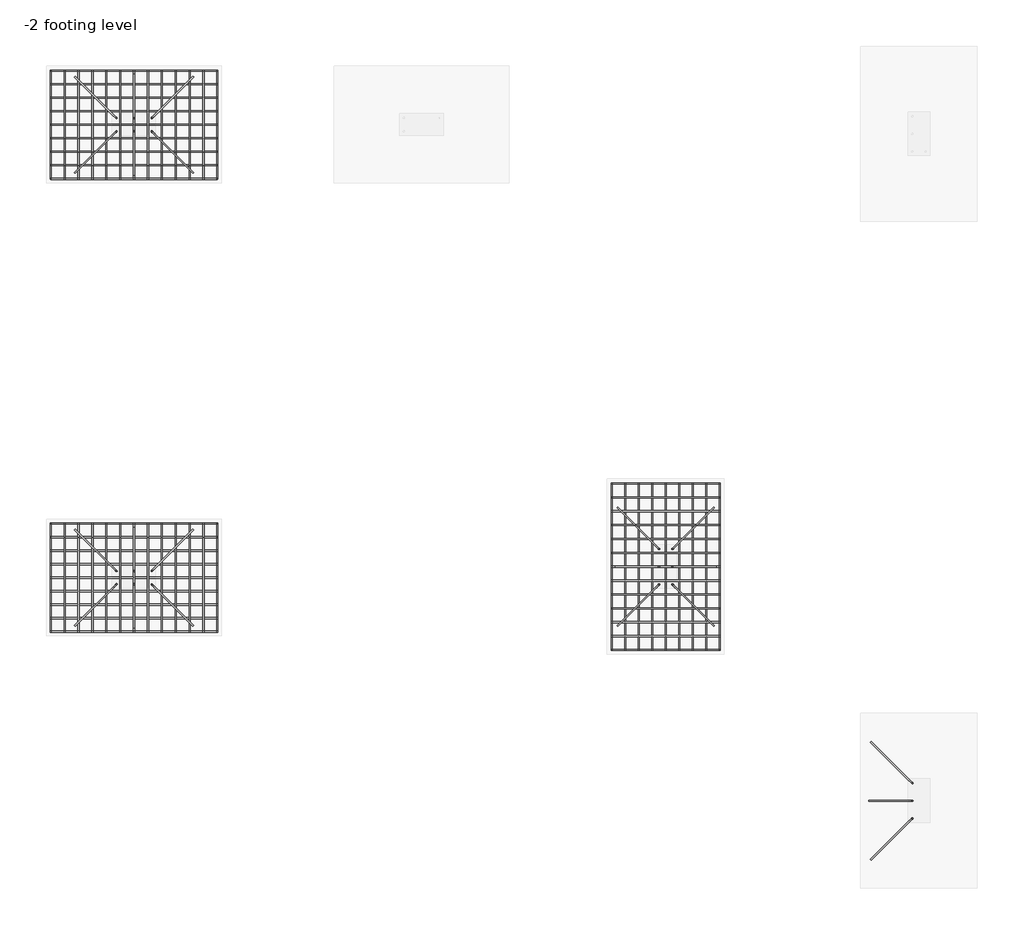
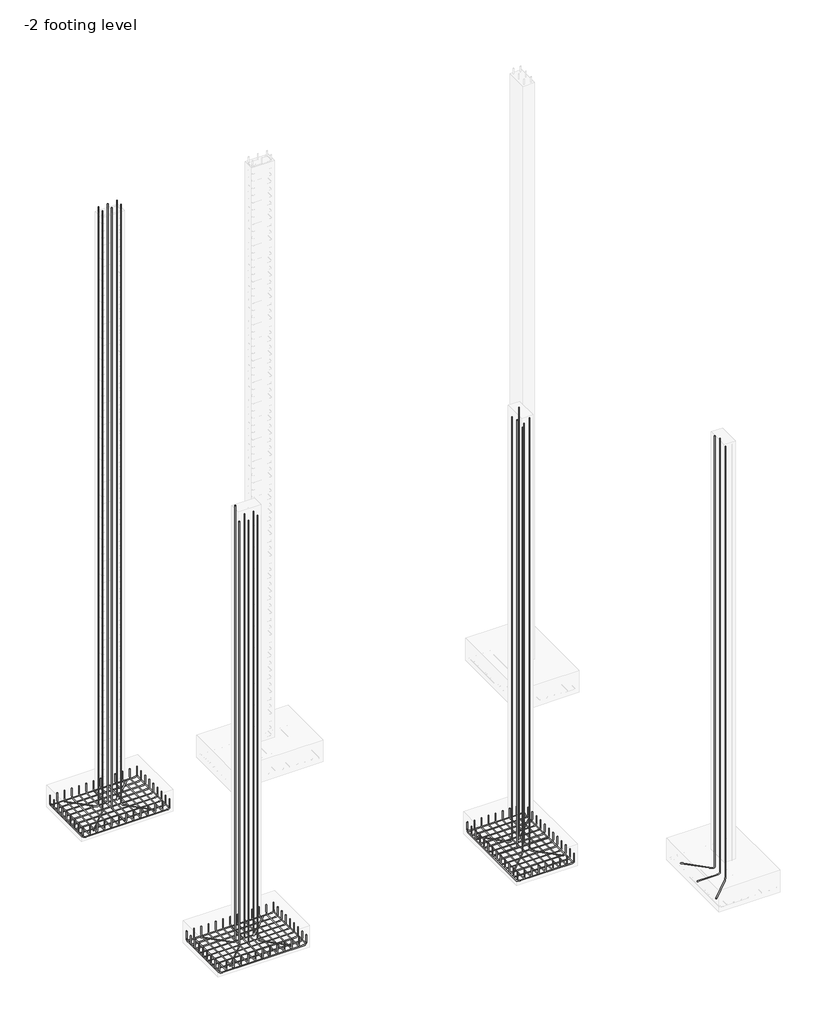
# One storey, part 2 of 9: 27 reinforcing bars.
"""IFC4 building model written with IfcOpenShell, lengths in millimetres."""

from ifc_helpers import new_model, si_unit, point, frame, origin, place, context, project, spatial, polyline, circle_curve, trimmed, segment, composite_curve, source, transform, mapped, element, save
from ifc_brep_helpers import swept_disk

model = new_model("IFC4")

# Units and contexts
model_context = context("Model", 3, world=origin())
ifc_project = project(units=[si_unit("LENGTHUNIT", "METRE", prefix="MILLI")], contexts=[model_context])

# Site, building, storey
site = spatial("IfcSite", under=ifc_project)
building = spatial("IfcBuilding", under=site)
storey = spatial("IfcBuildingStorey", under=building, Name="-2 footing level", Elevation=-1828.8)

# Reinforcing bars
placement = place(None, origin())
reinforcing_bar_shape = source(origin(), model_context, "Body", "SolidModel", [
    swept_disk(composite_curve([segment(polyline([(-7085.5501466, -1961.0445725, -2044.7), (-7085.5501466, -1961.0445725, -2197.1)]), True, "CONTINUOUS"), segment(trimmed(circle_curve(frame((-7130.0001466, -1961.0445725, -2197.1), z_axis=(0.0, 1.0, 0.0), x_axis=(44.45000000000073, 0.0, 0.0)), 44.45), [point((-7085.5501466, -1961.0445725, -2197.1))], [point((-7130.0001466, -1961.0445725, -2241.55))], True, "CARTESIAN"), True, "CONTINUOUS"), segment(polyline([(-7130.0001466, -1961.0445725, -2241.55), (-8781.0001466, -1961.0445725, -2241.55)]), True, "CONTINUOUS"), segment(trimmed(circle_curve(frame((-8781.0001466, -1961.0445725, -2197.1), z_axis=(0.0, 1.0, 0.0), x_axis=(0.0, 0.0, -44.45000000000027)), 44.45), [point((-8781.0001466, -1961.0445725, -2241.55))], [point((-8825.4501466, -1961.0445725, -2197.1))], True, "CARTESIAN"), True, "CONTINUOUS"), segment(polyline([(-8825.4501466, -1961.0445725, -2197.1), (-8825.4501466, -1961.0445725, -2044.7)]), True, "CONTINUOUS")], self_intersect=False), 6.35),
])
element("IfcReinforcingBar", 1, at=placement, inside=storey, context=model_context, shape_type="MappedRepresentation", body=[
    mapped(reinforcing_bar_shape, transform((0.0, 0.0, 0.0), x_axis=(1.0, 0.0, 0.0), y_axis=(0.0, 1.0, 0.0), z_axis=(0.0, 0.0, 1.0))),
    mapped(reinforcing_bar_shape, transform((0.0, -141.2875, 0.0), x_axis=(1.0, 0.0, 0.0), y_axis=(0.0, 1.0, 0.0), z_axis=(0.0, 0.0, 1.0))),
    mapped(reinforcing_bar_shape, transform((0.0, -282.575, 0.0), x_axis=(1.0, 0.0, 0.0), y_axis=(0.0, 1.0, 0.0), z_axis=(0.0, 0.0, 1.0))),
    mapped(reinforcing_bar_shape, transform((0.0, -423.8625, 0.0), x_axis=(1.0, 0.0, 0.0), y_axis=(0.0, 1.0, 0.0), z_axis=(0.0, 0.0, 1.0))),
    mapped(reinforcing_bar_shape, transform((0.0, -565.15, 0.0), x_axis=(1.0, 0.0, 0.0), y_axis=(0.0, 1.0, 0.0), z_axis=(0.0, 0.0, 1.0))),
    mapped(reinforcing_bar_shape, transform((0.0, -706.4375, 0.0), x_axis=(1.0, 0.0, 0.0), y_axis=(0.0, 1.0, 0.0), z_axis=(0.0, 0.0, 1.0))),
    mapped(reinforcing_bar_shape, transform((0.0, -847.725, 0.0), x_axis=(1.0, 0.0, 0.0), y_axis=(0.0, 1.0, 0.0), z_axis=(0.0, 0.0, 1.0))),
    mapped(reinforcing_bar_shape, transform((0.0, -989.0125, 0.0), x_axis=(1.0, 0.0, 0.0), y_axis=(0.0, 1.0, 0.0), z_axis=(0.0, 0.0, 1.0))),
    mapped(reinforcing_bar_shape, transform((0.0, -1130.3, 0.0), x_axis=(1.0, 0.0, 0.0), y_axis=(0.0, 1.0, 0.0), z_axis=(0.0, 0.0, 1.0))),
])
reinforcing_bar_2_shape = source(origin(), model_context, "Body", "SolidModel", [
    swept_disk(composite_curve([segment(polyline([(-8825.4501466, -1961.0445725, -2033.4041416), (-8825.4501466, -1961.0445725, -2185.8041416)]), True, "CONTINUOUS"), segment(trimmed(circle_curve(frame((-8825.4501466, -2005.4945725, -2185.8041416), z_axis=(-1.0, 0.0, 0.0), x_axis=(0.0, 44.450000000000045, 0.0)), 44.45), [point((-8825.4501466, -1961.0445725, -2185.8041416))], [point((-8825.4501466, -2005.4945725, -2230.2541416))], True, "CARTESIAN"), True, "CONTINUOUS"), segment(polyline([(-8825.4501466, -2005.4945725, -2230.2541416), (-8825.4501466, -3046.8945725, -2230.2541416)]), True, "CONTINUOUS"), segment(trimmed(circle_curve(frame((-8825.4501466, -3046.8945725, -2185.8041416), z_axis=(-1.0, 0.0, 0.0), x_axis=(0.0, 0.0, -44.44999999999982)), 44.45), [point((-8825.4501466, -3046.8945725, -2230.2541416))], [point((-8825.4501466, -3091.3445725, -2185.8041416))], True, "CARTESIAN"), True, "CONTINUOUS"), segment(polyline([(-8825.4501466, -3091.3445725, -2185.8041416), (-8825.4501466, -3091.3445725, -2033.4041416)]), True, "CONTINUOUS")], self_intersect=False), 6.35),
])
element("IfcReinforcingBar", 2, at=placement, inside=storey, context=model_context, shape_type="MappedRepresentation", body=[
    mapped(reinforcing_bar_2_shape, transform((0.0, 0.0, 0.0), x_axis=(1.0, 0.0, 0.0), y_axis=(0.0, 1.0, 0.0), z_axis=(0.0, 0.0, 1.0))),
    mapped(reinforcing_bar_2_shape, transform((144.9916667, 0.0, 0.0), x_axis=(1.0, 0.0, 0.0), y_axis=(0.0, 1.0, 0.0), z_axis=(0.0, 0.0, 1.0))),
    mapped(reinforcing_bar_2_shape, transform((289.9833333, 0.0, 0.0), x_axis=(1.0, 0.0, 0.0), y_axis=(0.0, 1.0, 0.0), z_axis=(0.0, 0.0, 1.0))),
    mapped(reinforcing_bar_2_shape, transform((434.975, 0.0, 0.0), x_axis=(1.0, 0.0, 0.0), y_axis=(0.0, 1.0, 0.0), z_axis=(0.0, 0.0, 1.0))),
    mapped(reinforcing_bar_2_shape, transform((579.9666667, 0.0, 0.0), x_axis=(1.0, 0.0, 0.0), y_axis=(0.0, 1.0, 0.0), z_axis=(0.0, 0.0, 1.0))),
    mapped(reinforcing_bar_2_shape, transform((724.9583333, 0.0, 0.0), x_axis=(1.0, 0.0, 0.0), y_axis=(0.0, 1.0, 0.0), z_axis=(0.0, 0.0, 1.0))),
    mapped(reinforcing_bar_2_shape, transform((869.95, 0.0, 0.0), x_axis=(1.0, 0.0, 0.0), y_axis=(0.0, 1.0, 0.0), z_axis=(0.0, 0.0, 1.0))),
    mapped(reinforcing_bar_2_shape, transform((1014.9416667, 0.0, 0.0), x_axis=(1.0, 0.0, 0.0), y_axis=(0.0, 1.0, 0.0), z_axis=(0.0, 0.0, 1.0))),
    mapped(reinforcing_bar_2_shape, transform((1159.9333333, 0.0, 0.0), x_axis=(1.0, 0.0, 0.0), y_axis=(0.0, 1.0, 0.0), z_axis=(0.0, 0.0, 1.0))),
    mapped(reinforcing_bar_2_shape, transform((1304.925, 0.0, 0.0), x_axis=(1.0, 0.0, 0.0), y_axis=(0.0, 1.0, 0.0), z_axis=(0.0, 0.0, 1.0))),
    mapped(reinforcing_bar_2_shape, transform((1449.9166667, 0.0, 0.0), x_axis=(1.0, 0.0, 0.0), y_axis=(0.0, 1.0, 0.0), z_axis=(0.0, 0.0, 1.0))),
    mapped(reinforcing_bar_2_shape, transform((1594.9083333, 0.0, 0.0), x_axis=(1.0, 0.0, 0.0), y_axis=(0.0, 1.0, 0.0), z_axis=(0.0, 0.0, 1.0))),
    mapped(reinforcing_bar_2_shape, transform((1739.9, 0.0, 0.0), x_axis=(1.0, 0.0, 0.0), y_axis=(0.0, 1.0, 0.0), z_axis=(0.0, 0.0, 1.0))),
])
reinforcing_bar_3_shape = source(origin(), model_context, "Body", "SolidModel", [
    swept_disk(composite_curve([segment(polyline([(-8825.4501466, -7824.8766794, -2044.7), (-8825.4501466, -7824.8766794, -2197.1)]), True, "CONTINUOUS"), segment(trimmed(circle_curve(frame((-8781.0001466, -7824.8766794, -2197.1), z_axis=(0.0, -1.0, 0.0), x_axis=(-44.45000000000073, 0.0, 0.0)), 44.45), [point((-8825.4501466, -7824.8766794, -2197.1))], [point((-8781.0001466, -7824.8766794, -2241.55))], True, "CARTESIAN"), True, "CONTINUOUS"), segment(polyline([(-8781.0001466, -7824.8766794, -2241.55), (-7130.0001466, -7824.8766794, -2241.55)]), True, "CONTINUOUS"), segment(trimmed(circle_curve(frame((-7130.0001466, -7824.8766794, -2197.1), z_axis=(0.0, -1.0, 0.0), x_axis=(0.0, 0.0, -44.45000000000027)), 44.45), [point((-7130.0001466, -7824.8766794, -2241.55))], [point((-7085.5501466, -7824.8766794, -2197.1))], True, "CARTESIAN"), True, "CONTINUOUS"), segment(polyline([(-7085.5501466, -7824.8766794, -2197.1), (-7085.5501466, -7824.8766794, -2044.7)]), True, "CONTINUOUS")], self_intersect=False), 6.35),
])
element("IfcReinforcingBar", 3, at=placement, inside=storey, context=model_context, shape_type="MappedRepresentation", body=[
    mapped(reinforcing_bar_3_shape, transform((0.0, 0.0, 0.0), x_axis=(1.0, 0.0, 0.0), y_axis=(0.0, 1.0, 0.0), z_axis=(0.0, 0.0, 1.0))),
    mapped(reinforcing_bar_3_shape, transform((0.0, 141.2875, 0.0), x_axis=(1.0, 0.0, 0.0), y_axis=(0.0, 1.0, 0.0), z_axis=(0.0, 0.0, 1.0))),
    mapped(reinforcing_bar_3_shape, transform((0.0, 282.575, 0.0), x_axis=(1.0, 0.0, 0.0), y_axis=(0.0, 1.0, 0.0), z_axis=(0.0, 0.0, 1.0))),
    mapped(reinforcing_bar_3_shape, transform((0.0, 423.8625, 0.0), x_axis=(1.0, 0.0, 0.0), y_axis=(0.0, 1.0, 0.0), z_axis=(0.0, 0.0, 1.0))),
    mapped(reinforcing_bar_3_shape, transform((0.0, 565.15, 0.0), x_axis=(1.0, 0.0, 0.0), y_axis=(0.0, 1.0, 0.0), z_axis=(0.0, 0.0, 1.0))),
    mapped(reinforcing_bar_3_shape, transform((0.0, 706.4375, 0.0), x_axis=(1.0, 0.0, 0.0), y_axis=(0.0, 1.0, 0.0), z_axis=(0.0, 0.0, 1.0))),
    mapped(reinforcing_bar_3_shape, transform((0.0, 847.725, 0.0), x_axis=(1.0, 0.0, 0.0), y_axis=(0.0, 1.0, 0.0), z_axis=(0.0, 0.0, 1.0))),
    mapped(reinforcing_bar_3_shape, transform((0.0, 989.0125, 0.0), x_axis=(1.0, 0.0, 0.0), y_axis=(0.0, 1.0, 0.0), z_axis=(0.0, 0.0, 1.0))),
    mapped(reinforcing_bar_3_shape, transform((0.0, 1130.3, 0.0), x_axis=(1.0, 0.0, 0.0), y_axis=(0.0, 1.0, 0.0), z_axis=(0.0, 0.0, 1.0))),
])
reinforcing_bar_4_shape = source(origin(), model_context, "Body", "SolidModel", [
    swept_disk(composite_curve([segment(polyline([(-7085.5501466, -7824.8766794, -2033.4041416), (-7085.5501466, -7824.8766794, -2185.8041416)]), True, "CONTINUOUS"), segment(trimmed(circle_curve(frame((-7085.5501466, -7780.4266794, -2185.8041416), z_axis=(1.0, 0.0, 0.0), x_axis=(0.0, -44.45000000000073, 0.0)), 44.45), [point((-7085.5501466, -7824.8766794, -2185.8041416))], [point((-7085.5501466, -7780.4266794, -2230.2541416))], True, "CARTESIAN"), True, "CONTINUOUS"), segment(polyline([(-7085.5501466, -7780.4266794, -2230.2541416), (-7085.5501466, -6739.0266794, -2230.2541416)]), True, "CONTINUOUS"), segment(trimmed(circle_curve(frame((-7085.5501466, -6739.0266794, -2185.8041416), z_axis=(1.0, 0.0, 0.0), x_axis=(0.0, 0.0, -44.44999999999982)), 44.45), [point((-7085.5501466, -6739.0266794, -2230.2541416))], [point((-7085.5501466, -6694.5766794, -2185.8041416))], True, "CARTESIAN"), True, "CONTINUOUS"), segment(polyline([(-7085.5501466, -6694.5766794, -2185.8041416), (-7085.5501466, -6694.5766794, -2033.4041416)]), True, "CONTINUOUS")], self_intersect=False), 6.35),
])
element("IfcReinforcingBar", 4, at=placement, inside=storey, context=model_context, shape_type="MappedRepresentation", body=[
    mapped(reinforcing_bar_4_shape, transform((0.0, 0.0, 0.0), x_axis=(1.0, 0.0, 0.0), y_axis=(0.0, 1.0, 0.0), z_axis=(0.0, 0.0, 1.0))),
    mapped(reinforcing_bar_4_shape, transform((-144.9916667, 0.0, 0.0), x_axis=(1.0, 0.0, 0.0), y_axis=(0.0, 1.0, 0.0), z_axis=(0.0, 0.0, 1.0))),
    mapped(reinforcing_bar_4_shape, transform((-289.9833333, 0.0, 0.0), x_axis=(1.0, 0.0, 0.0), y_axis=(0.0, 1.0, 0.0), z_axis=(0.0, 0.0, 1.0))),
    mapped(reinforcing_bar_4_shape, transform((-434.975, 0.0, 0.0), x_axis=(1.0, 0.0, 0.0), y_axis=(0.0, 1.0, 0.0), z_axis=(0.0, 0.0, 1.0))),
    mapped(reinforcing_bar_4_shape, transform((-579.9666667, 0.0, 0.0), x_axis=(1.0, 0.0, 0.0), y_axis=(0.0, 1.0, 0.0), z_axis=(0.0, 0.0, 1.0))),
    mapped(reinforcing_bar_4_shape, transform((-724.9583333, 0.0, 0.0), x_axis=(1.0, 0.0, 0.0), y_axis=(0.0, 1.0, 0.0), z_axis=(0.0, 0.0, 1.0))),
    mapped(reinforcing_bar_4_shape, transform((-869.95, 0.0, 0.0), x_axis=(1.0, 0.0, 0.0), y_axis=(0.0, 1.0, 0.0), z_axis=(0.0, 0.0, 1.0))),
    mapped(reinforcing_bar_4_shape, transform((-1014.9416667, 0.0, 0.0), x_axis=(1.0, 0.0, 0.0), y_axis=(0.0, 1.0, 0.0), z_axis=(0.0, 0.0, 1.0))),
    mapped(reinforcing_bar_4_shape, transform((-1159.9333333, 0.0, 0.0), x_axis=(1.0, 0.0, 0.0), y_axis=(0.0, 1.0, 0.0), z_axis=(0.0, 0.0, 1.0))),
    mapped(reinforcing_bar_4_shape, transform((-1304.925, 0.0, 0.0), x_axis=(1.0, 0.0, 0.0), y_axis=(0.0, 1.0, 0.0), z_axis=(0.0, 0.0, 1.0))),
    mapped(reinforcing_bar_4_shape, transform((-1449.9166667, 0.0, 0.0), x_axis=(1.0, 0.0, 0.0), y_axis=(0.0, 1.0, 0.0), z_axis=(0.0, 0.0, 1.0))),
    mapped(reinforcing_bar_4_shape, transform((-1594.9083333, 0.0, 0.0), x_axis=(1.0, 0.0, 0.0), y_axis=(0.0, 1.0, 0.0), z_axis=(0.0, 0.0, 1.0))),
    mapped(reinforcing_bar_4_shape, transform((-1739.9, 0.0, 0.0), x_axis=(1.0, 0.0, 0.0), y_axis=(0.0, 1.0, 0.0), z_axis=(0.0, 0.0, 1.0))),
])
reinforcing_bar_5_shape = source(origin(), model_context, "Body", "SolidModel", [
    swept_disk(composite_curve([segment(polyline([(-2967.3323872, -6275.4766794, -2044.7), (-2967.3323872, -6275.4766794, -2197.1)]), True, "CONTINUOUS"), segment(trimmed(circle_curve(frame((-2967.3323872, -6319.9266794, -2197.1), z_axis=(-1.0, 0.0, 0.0), x_axis=(0.0, 44.44999999999982, 0.0)), 44.45), [point((-2967.3323872, -6275.4766794, -2197.1))], [point((-2967.3323872, -6319.9266794, -2241.55))], True, "CARTESIAN"), True, "CONTINUOUS"), segment(polyline([(-2967.3323872, -6319.9266794, -2241.55), (-2967.3323872, -7970.9266794, -2241.55)]), True, "CONTINUOUS"), segment(trimmed(circle_curve(frame((-2967.3323872, -7970.9266794, -2197.1), z_axis=(-1.0, 0.0, 0.0), x_axis=(0.0, 0.0, -44.45000000000027)), 44.45), [point((-2967.3323872, -7970.9266794, -2241.55))], [point((-2967.3323872, -8015.3766794, -2197.1))], True, "CARTESIAN"), True, "CONTINUOUS"), segment(polyline([(-2967.3323872, -8015.3766794, -2197.1), (-2967.3323872, -8015.3766794, -2044.7)]), True, "CONTINUOUS")], self_intersect=False), 6.35),
])
element("IfcReinforcingBar", 5, at=placement, inside=storey, context=model_context, shape_type="MappedRepresentation", body=[
    mapped(reinforcing_bar_5_shape, transform((0.0, 0.0, 0.0), x_axis=(1.0, 0.0, 0.0), y_axis=(0.0, 1.0, 0.0), z_axis=(0.0, 0.0, 1.0))),
    mapped(reinforcing_bar_5_shape, transform((141.2875, 0.0, 0.0), x_axis=(1.0, 0.0, 0.0), y_axis=(0.0, 1.0, 0.0), z_axis=(0.0, 0.0, 1.0))),
    mapped(reinforcing_bar_5_shape, transform((282.575, 0.0, 0.0), x_axis=(1.0, 0.0, 0.0), y_axis=(0.0, 1.0, 0.0), z_axis=(0.0, 0.0, 1.0))),
    mapped(reinforcing_bar_5_shape, transform((423.8625, 0.0, 0.0), x_axis=(1.0, 0.0, 0.0), y_axis=(0.0, 1.0, 0.0), z_axis=(0.0, 0.0, 1.0))),
    mapped(reinforcing_bar_5_shape, transform((565.15, 0.0, 0.0), x_axis=(1.0, 0.0, 0.0), y_axis=(0.0, 1.0, 0.0), z_axis=(0.0, 0.0, 1.0))),
    mapped(reinforcing_bar_5_shape, transform((706.4375, 0.0, 0.0), x_axis=(1.0, 0.0, 0.0), y_axis=(0.0, 1.0, 0.0), z_axis=(0.0, 0.0, 1.0))),
    mapped(reinforcing_bar_5_shape, transform((847.725, 0.0, 0.0), x_axis=(1.0, 0.0, 0.0), y_axis=(0.0, 1.0, 0.0), z_axis=(0.0, 0.0, 1.0))),
    mapped(reinforcing_bar_5_shape, transform((989.0125, 0.0, 0.0), x_axis=(1.0, 0.0, 0.0), y_axis=(0.0, 1.0, 0.0), z_axis=(0.0, 0.0, 1.0))),
    mapped(reinforcing_bar_5_shape, transform((1130.3, 0.0, 0.0), x_axis=(1.0, 0.0, 0.0), y_axis=(0.0, 1.0, 0.0), z_axis=(0.0, 0.0, 1.0))),
])
reinforcing_bar_6_shape = source(origin(), model_context, "Body", "SolidModel", [
    swept_disk(composite_curve([segment(polyline([(-2967.3323872, -8015.3766794, -2033.4041416), (-2967.3323872, -8015.3766794, -2185.8041416)]), True, "CONTINUOUS"), segment(trimmed(circle_curve(frame((-2922.8823872, -8015.3766794, -2185.8041416), z_axis=(0.0, -1.0, 0.0), x_axis=(-44.45000000000027, 0.0, 0.0)), 44.45), [point((-2967.3323872, -8015.3766794, -2185.8041416))], [point((-2922.8823872, -8015.3766794, -2230.2541416))], True, "CARTESIAN"), True, "CONTINUOUS"), segment(polyline([(-2922.8823872, -8015.3766794, -2230.2541416), (-1881.4823872, -8015.3766794, -2230.2541416)]), True, "CONTINUOUS"), segment(trimmed(circle_curve(frame((-1881.4823872, -8015.3766794, -2185.8041416), z_axis=(0.0, -1.0, 0.0), x_axis=(0.0, 0.0, -44.44999999999982)), 44.45), [point((-1881.4823872, -8015.3766794, -2230.2541416))], [point((-1837.0323872, -8015.3766794, -2185.8041416))], True, "CARTESIAN"), True, "CONTINUOUS"), segment(polyline([(-1837.0323872, -8015.3766794, -2185.8041416), (-1837.0323872, -8015.3766794, -2033.4041416)]), True, "CONTINUOUS")], self_intersect=False), 6.35),
])
element("IfcReinforcingBar", 6, at=placement, inside=storey, context=model_context, shape_type="MappedRepresentation", body=[
    mapped(reinforcing_bar_6_shape, transform((0.0, 0.0, 0.0), x_axis=(1.0, 0.0, 0.0), y_axis=(0.0, 1.0, 0.0), z_axis=(0.0, 0.0, 1.0))),
    mapped(reinforcing_bar_6_shape, transform((0.0, 144.9916667, 0.0), x_axis=(1.0, 0.0, 0.0), y_axis=(0.0, 1.0, 0.0), z_axis=(0.0, 0.0, 1.0))),
    mapped(reinforcing_bar_6_shape, transform((0.0, 289.9833333, 0.0), x_axis=(1.0, 0.0, 0.0), y_axis=(0.0, 1.0, 0.0), z_axis=(0.0, 0.0, 1.0))),
    mapped(reinforcing_bar_6_shape, transform((0.0, 434.975, 0.0), x_axis=(1.0, 0.0, 0.0), y_axis=(0.0, 1.0, 0.0), z_axis=(0.0, 0.0, 1.0))),
    mapped(reinforcing_bar_6_shape, transform((0.0, 579.9666667, 0.0), x_axis=(1.0, 0.0, 0.0), y_axis=(0.0, 1.0, 0.0), z_axis=(0.0, 0.0, 1.0))),
    mapped(reinforcing_bar_6_shape, transform((0.0, 724.9583333, 0.0), x_axis=(1.0, 0.0, 0.0), y_axis=(0.0, 1.0, 0.0), z_axis=(0.0, 0.0, 1.0))),
    mapped(reinforcing_bar_6_shape, transform((0.0, 869.95, 0.0), x_axis=(1.0, 0.0, 0.0), y_axis=(0.0, 1.0, 0.0), z_axis=(0.0, 0.0, 1.0))),
    mapped(reinforcing_bar_6_shape, transform((0.0, 1014.9416667, 0.0), x_axis=(1.0, 0.0, 0.0), y_axis=(0.0, 1.0, 0.0), z_axis=(0.0, 0.0, 1.0))),
    mapped(reinforcing_bar_6_shape, transform((0.0, 1159.9333333, 0.0), x_axis=(1.0, 0.0, 0.0), y_axis=(0.0, 1.0, 0.0), z_axis=(0.0, 0.0, 1.0))),
    mapped(reinforcing_bar_6_shape, transform((0.0, 1304.925, 0.0), x_axis=(1.0, 0.0, 0.0), y_axis=(0.0, 1.0, 0.0), z_axis=(0.0, 0.0, 1.0))),
    mapped(reinforcing_bar_6_shape, transform((0.0, 1449.9166667, 0.0), x_axis=(1.0, 0.0, 0.0), y_axis=(0.0, 1.0, 0.0), z_axis=(0.0, 0.0, 1.0))),
    mapped(reinforcing_bar_6_shape, transform((0.0, 1594.9083333, 0.0), x_axis=(1.0, 0.0, 0.0), y_axis=(0.0, 1.0, 0.0), z_axis=(0.0, 0.0, 1.0))),
    mapped(reinforcing_bar_6_shape, transform((0.0, 1739.9, 0.0), x_axis=(1.0, 0.0, 0.0), y_axis=(0.0, 1.0, 0.0), z_axis=(0.0, 0.0, 1.0))),
])
element("IfcReinforcingBar", 7, at=placement, inside=storey, context=model_context, shape_type="SolidModel", body=[
    swept_disk(composite_curve([segment(polyline([(-259.3446547, -10209.1829565, -2212.9582082), (142.6779331, -9807.1603688, -2212.9582082)]), True, "CONTINUOUS"), segment(trimmed(circle_curve(frame((142.6779331, -9807.1603688, -2168.5082082), z_axis=(0.7071067811865501, -0.7071067811865449, 0.0), x_axis=(0.0, 0.0, -44.45000000000027)), 44.45), [point((142.6779331, -9807.1603688, -2212.9582082))], [point((174.1088295, -9775.7294723, -2168.5082082))], True, "CARTESIAN"), True, "CONTINUOUS"), segment(polyline([(174.1088295, -9775.7294723, -2168.5082082), (174.1088295, -9775.7294723, 6931.0417918)]), True, "CONTINUOUS")], self_intersect=False), 6.35),
])
element("IfcReinforcingBar", 8, at=placement, inside=storey, context=model_context, shape_type="SolidModel", body=[
    swept_disk(composite_curve([segment(polyline([(-259.3446547, -8973.9759881, -2212.9582082), (142.6779331, -9375.9985759, -2212.9582082)]), True, "CONTINUOUS"), segment(trimmed(circle_curve(frame((142.6779331, -9375.9985759, -2168.5082082), z_axis=(-0.7071067811865501, -0.7071067811865449, 0.0), x_axis=(0.0, 0.0, -44.45000000000027)), 44.45), [point((142.6779331, -9375.9985759, -2212.9582082))], [point((174.1088295, -9407.4294723, -2168.5082082))], True, "CARTESIAN"), True, "CONTINUOUS"), segment(polyline([(174.1088295, -9407.4294723, -2168.5082082), (174.1088295, -9407.4294723, 6931.0417918)]), True, "CONTINUOUS")], self_intersect=False), 6.35),
])
element("IfcReinforcingBar", 9, at=placement, inside=storey, context=model_context, shape_type="SolidModel", body=[
    swept_disk(composite_curve([segment(polyline([(-283.0911705, -9591.5794723, -2212.9582082), (129.6588295, -9591.5794723, -2212.9582082)]), True, "CONTINUOUS"), segment(trimmed(circle_curve(frame((129.6588295, -9591.5794723, -2168.5082082), z_axis=(0.0, -1.0, 0.0), x_axis=(0.0, 0.0, -44.45000000000027)), 44.45), [point((129.6588295, -9591.5794723, -2212.9582082))], [point((174.1088295, -9591.5794723, -2168.5082082))], True, "CARTESIAN"), True, "CONTINUOUS"), segment(polyline([(174.1088295, -9591.5794723, -2168.5082082), (174.1088295, -9591.5794723, 6988.1917918)]), True, "CONTINUOUS")], self_intersect=False), 6.35),
])
element("IfcReinforcingBar", 10, at=placement, inside=storey, context=model_context, shape_type="SolidModel", body=[
    swept_disk(composite_curve([segment(polyline([(-8573.7058773, -6756.4231952, -2212.9582082), (-8171.0810431, -7159.0480295, -2212.9582082)]), True, "CONTINUOUS"), segment(trimmed(circle_curve(frame((-8171.0810431, -7159.0480295, -2168.5082082), z_axis=(-0.7071067811865455, -0.7071067811865496, 0.0), x_axis=(0.0, 0.0, -44.45000000000027)), 44.45), [point((-8171.0810431, -7159.0480295, -2212.9582082))], [point((-8139.6501466, -7190.4789259, -2168.5082082))], True, "CARTESIAN"), True, "CONTINUOUS"), segment(polyline([(-8139.6501466, -7190.4789259, -2168.5082082), (-8139.6501466, -7190.4789259, 7033.7249395)]), True, "CONTINUOUS")], self_intersect=False), 6.35),
])
element("IfcReinforcingBar", 11, at=placement, inside=storey, context=model_context, shape_type="SolidModel", body=[
    swept_disk(composite_curve([segment(polyline([(-8573.7058773, -7763.0301636, -2212.9582082), (-8171.0810431, -7360.4053294, -2212.9582082)]), True, "CONTINUOUS"), segment(trimmed(circle_curve(frame((-8171.0810431, -7360.4053294, -2168.5082082), z_axis=(0.707106781186541, -0.707106781186554, 0.0), x_axis=(0.0, 0.0, -44.45000000000027)), 44.45), [point((-8171.0810431, -7360.4053294, -2212.9582082))], [point((-8139.6501466, -7328.974433, -2168.5082082))], True, "CARTESIAN"), True, "CONTINUOUS"), segment(polyline([(-8139.6501466, -7328.974433, -2168.5082082), (-8139.6501466, -7328.974433, 6778.6417918)]), True, "CONTINUOUS")], self_intersect=False), 6.35),
])
element("IfcReinforcingBar", 12, at=placement, inside=storey, context=model_context, shape_type="SolidModel", body=[
    swept_disk(composite_curve([segment(polyline([(-7338.4989089, -6756.4231952, -2212.9582082), (-7740.5214967, -7158.445783, -2212.9582082)]), True, "CONTINUOUS"), segment(trimmed(circle_curve(frame((-7740.5214967, -7158.445783, -2168.5082082), z_axis=(-0.7071067811865444, 0.7071067811865507, 0.0), x_axis=(0.0, 0.0, -44.45000000000027)), 44.45), [point((-7740.5214967, -7158.445783, -2212.9582082))], [point((-7771.9523931, -7189.8766794, -2168.5082082))], True, "CARTESIAN"), True, "CONTINUOUS"), segment(polyline([(-7771.9523931, -7189.8766794, -2168.5082082), (-7771.9523931, -7189.8766794, 6778.6417918)]), True, "CONTINUOUS")], self_intersect=False), 6.35),
])
element("IfcReinforcingBar", 13, at=placement, inside=storey, context=model_context, shape_type="SolidModel", body=[
    swept_disk(composite_curve([segment(polyline([(-7338.4989089, -7763.0301636, -2212.9582082), (-7740.5214967, -7361.0075759, -2212.9582082)]), True, "CONTINUOUS"), segment(trimmed(circle_curve(frame((-7740.5214967, -7361.0075759, -2168.5082082), z_axis=(0.7071067811865421, 0.7071067811865529, 0.0), x_axis=(0.0, 0.0, -44.45000000000027)), 44.45), [point((-7740.5214967, -7361.0075759, -2212.9582082))], [point((-7771.9523931, -7329.5766794, -2168.5082082))], True, "CARTESIAN"), True, "CONTINUOUS"), segment(polyline([(-7771.9523931, -7329.5766794, -2168.5082082), (-7771.9523931, -7329.5766794, 6778.6417918)]), True, "CONTINUOUS")], self_intersect=False), 6.35),
])
element("IfcReinforcingBar", 14, at=placement, inside=storey, context=model_context, shape_type="SolidModel", body=[
    swept_disk(composite_curve([segment(polyline([(-7956.1023931, -6732.6766794, -2212.9582082), (-7956.1023931, -7146.8157419, -2212.9582082)]), True, "CONTINUOUS"), segment(trimmed(circle_curve(frame((-7956.1023931, -7146.8157419, -2168.5082082), z_axis=(-1.0, 0.0, 0.0), x_axis=(0.0, 0.0, -44.45000000000027)), 44.45), [point((-7956.1023931, -7146.8157419, -2212.9582082))], [point((-7956.1023931, -7191.2657419, -2168.5082082))], True, "CARTESIAN"), True, "CONTINUOUS"), segment(polyline([(-7956.1023931, -7191.2657419, -2168.5082082), (-7956.1023931, -7191.2657419, 6785.4844027)]), True, "CONTINUOUS")], self_intersect=False), 6.35),
])
element("IfcReinforcingBar", 15, at=placement, inside=storey, context=model_context, shape_type="SolidModel", body=[
    swept_disk(composite_curve([segment(polyline([(-7956.1023931, -7786.7766794, -2212.9582082), (-7956.1023931, -7372.6376169, -2212.9582082)]), True, "CONTINUOUS"), segment(trimmed(circle_curve(frame((-7956.1023931, -7372.6376169, -2168.5082082), z_axis=(1.0, 0.0, 0.0), x_axis=(0.0, 0.0, -44.45000000000027)), 44.45), [point((-7956.1023931, -7372.6376169, -2212.9582082))], [point((-7956.1023931, -7328.1876169, -2168.5082082))], True, "CARTESIAN"), True, "CONTINUOUS"), segment(polyline([(-7956.1023931, -7328.1876169, -2168.5082082), (-7956.1023931, -7328.1876169, 6730.1799535)]), True, "CONTINUOUS")], self_intersect=False), 6.35),
])
element("IfcReinforcingBar", 16, at=placement, inside=storey, context=model_context, shape_type="SolidModel", body=[
    swept_disk(composite_curve([segment(polyline([(-8573.7058773, -2022.8910883, -2212.9582082), (-8171.6832895, -2424.9136761, -2212.9582082)]), True, "CONTINUOUS"), segment(trimmed(circle_curve(frame((-8171.6832895, -2424.9136761, -2168.5082082), z_axis=(-0.7071067811865455, -0.7071067811865496, 0.0), x_axis=(0.0, 0.0, -44.45000000000027)), 44.45), [point((-8171.6832895, -2424.9136761, -2212.9582082))], [point((-8140.2523931, -2456.3445725, -2168.5082082))], True, "CARTESIAN"), True, "CONTINUOUS"), segment(polyline([(-8140.2523931, -2456.3445725, -2168.5082082), (-8140.2523931, -2456.3445725, 10477.5)]), True, "CONTINUOUS")], self_intersect=False), 6.35),
])
element("IfcReinforcingBar", 17, at=placement, inside=storey, context=model_context, shape_type="SolidModel", body=[
    swept_disk(composite_curve([segment(polyline([(-8573.7058773, -3029.4980567, -2212.9582082), (-8171.6832895, -2627.4754689, -2212.9582082)]), True, "CONTINUOUS"), segment(trimmed(circle_curve(frame((-8171.6832895, -2627.4754689, -2168.5082082), z_axis=(0.707106781186541, -0.707106781186554, 0.0), x_axis=(0.0, 0.0, -44.45000000000027)), 44.45), [point((-8171.6832895, -2627.4754689, -2212.9582082))], [point((-8140.2523931, -2596.0445725, -2168.5082082))], True, "CARTESIAN"), True, "CONTINUOUS"), segment(polyline([(-8140.2523931, -2596.0445725, -2168.5082082), (-8140.2523931, -2596.0445725, 10477.5)]), True, "CONTINUOUS")], self_intersect=False), 6.35),
])
element("IfcReinforcingBar", 18, at=placement, inside=storey, context=model_context, shape_type="SolidModel", body=[
    swept_disk(composite_curve([segment(polyline([(-7338.4989089, -2022.8910883, -2212.9582082), (-7740.5214967, -2424.9136761, -2212.9582082)]), True, "CONTINUOUS"), segment(trimmed(circle_curve(frame((-7740.5214967, -2424.9136761, -2168.5082082), z_axis=(-0.7071067811865444, 0.7071067811865507, 0.0), x_axis=(0.0, 0.0, -44.45000000000027)), 44.45), [point((-7740.5214967, -2424.9136761, -2212.9582082))], [point((-7771.9523931, -2456.3445725, -2168.5082082))], True, "CARTESIAN"), True, "CONTINUOUS"), segment(polyline([(-7771.9523931, -2456.3445725, -2168.5082082), (-7771.9523931, -2456.3445725, 10477.5)]), True, "CONTINUOUS")], self_intersect=False), 6.35),
])
element("IfcReinforcingBar", 19, at=placement, inside=storey, context=model_context, shape_type="SolidModel", body=[
    swept_disk(composite_curve([segment(polyline([(-7338.4989089, -3029.4980567, -2212.9582082), (-7740.5214967, -2627.4754689, -2212.9582082)]), True, "CONTINUOUS"), segment(trimmed(circle_curve(frame((-7740.5214967, -2627.4754689, -2168.5082082), z_axis=(0.7071067811865421, 0.7071067811865529, 0.0), x_axis=(0.0, 0.0, -44.45000000000027)), 44.45), [point((-7740.5214967, -2627.4754689, -2212.9582082))], [point((-7771.9523931, -2596.0445725, -2168.5082082))], True, "CARTESIAN"), True, "CONTINUOUS"), segment(polyline([(-7771.9523931, -2596.0445725, -2168.5082082), (-7771.9523931, -2596.0445725, 10477.5)]), True, "CONTINUOUS")], self_intersect=False), 6.35),
])
element("IfcReinforcingBar", 20, at=placement, inside=storey, context=model_context, shape_type="SolidModel", body=[
    swept_disk(composite_curve([segment(polyline([(-7956.1023931, -1999.1445725, -2212.9582082), (-7956.1023931, -2413.283635, -2212.9582082)]), True, "CONTINUOUS"), segment(trimmed(circle_curve(frame((-7956.1023931, -2413.283635, -2168.5082082), z_axis=(-1.0, 0.0, 0.0), x_axis=(0.0, 0.0, -44.45000000000027)), 44.45), [point((-7956.1023931, -2413.283635, -2212.9582082))], [point((-7956.1023931, -2457.733635, -2168.5082082))], True, "CARTESIAN"), True, "CONTINUOUS"), segment(polyline([(-7956.1023931, -2457.733635, -2168.5082082), (-7956.1023931, -2457.733635, 10477.5)]), True, "CONTINUOUS")], self_intersect=False), 6.35),
])
element("IfcReinforcingBar", 21, at=placement, inside=storey, context=model_context, shape_type="SolidModel", body=[
    swept_disk(composite_curve([segment(polyline([(-7956.1023931, -3053.2445725, -2212.9582082), (-7956.1023931, -2639.10551, -2212.9582082)]), True, "CONTINUOUS"), segment(trimmed(circle_curve(frame((-7956.1023931, -2639.10551, -2168.5082082), z_axis=(1.0, 0.0, 0.0), x_axis=(0.0, 0.0, -44.45000000000027)), 44.45), [point((-7956.1023931, -2639.10551, -2212.9582082))], [point((-7956.1023931, -2594.65551, -2168.5082082))], True, "CARTESIAN"), True, "CONTINUOUS"), segment(polyline([(-7956.1023931, -2594.65551, -2168.5082082), (-7956.1023931, -2594.65551, 10477.5)]), True, "CONTINUOUS")], self_intersect=False), 6.35),
])
element("IfcReinforcingBar", 22, at=placement, inside=storey, context=model_context, shape_type="SolidModel", body=[
    swept_disk(composite_curve([segment(polyline([(-2905.4858714, -7763.0301636, -2212.9582082), (-2503.4632836, -7361.0075759, -2212.9582082)]), True, "CONTINUOUS"), segment(trimmed(circle_curve(frame((-2503.4632836, -7361.0075759, -2168.5082082), z_axis=(0.7071067811865501, -0.7071067811865449, 0.0), x_axis=(0.0, 0.0, -44.45000000000027)), 44.45), [point((-2503.4632836, -7361.0075759, -2212.9582082))], [point((-2472.0323872, -7329.5766794, -2168.5082082))], True, "CARTESIAN"), True, "CONTINUOUS"), segment(polyline([(-2472.0323872, -7329.5766794, -2168.5082082), (-2472.0323872, -7329.5766794, 6778.6417918)]), True, "CONTINUOUS")], self_intersect=False), 6.35),
])
element("IfcReinforcingBar", 23, at=placement, inside=storey, context=model_context, shape_type="SolidModel", body=[
    swept_disk(composite_curve([segment(polyline([(-1898.878903, -7763.0301636, -2212.9582082), (-2300.9014908, -7361.0075759, -2212.9582082)]), True, "CONTINUOUS"), segment(trimmed(circle_curve(frame((-2300.9014908, -7361.0075759, -2168.5082082), z_axis=(0.7071067811865535, 0.7071067811865416, 0.0), x_axis=(0.0, 0.0, -44.45000000000027)), 44.45), [point((-2300.9014908, -7361.0075759, -2212.9582082))], [point((-2332.3323872, -7329.5766794, -2168.5082082))], True, "CARTESIAN"), True, "CONTINUOUS"), segment(polyline([(-2332.3323872, -7329.5766794, -2168.5082082), (-2332.3323872, -7329.5766794, 6931.0417918)]), True, "CONTINUOUS")], self_intersect=False), 6.35),
])
element("IfcReinforcingBar", 24, at=placement, inside=storey, context=model_context, shape_type="SolidModel", body=[
    swept_disk(composite_curve([segment(polyline([(-2905.4858714, -6527.8231952, -2212.9582082), (-2503.4632836, -6929.845783, -2212.9582082)]), True, "CONTINUOUS"), segment(trimmed(circle_curve(frame((-2503.4632836, -6929.845783, -2168.5082082), z_axis=(-0.7071067811865501, -0.7071067811865449, 0.0), x_axis=(0.0, 0.0, -44.45000000000027)), 44.45), [point((-2503.4632836, -6929.845783, -2212.9582082))], [point((-2472.0323872, -6961.2766794, -2168.5082082))], True, "CARTESIAN"), True, "CONTINUOUS"), segment(polyline([(-2472.0323872, -6961.2766794, -2168.5082082), (-2472.0323872, -6961.2766794, 6778.6417918)]), True, "CONTINUOUS")], self_intersect=False), 6.35),
])
element("IfcReinforcingBar", 25, at=placement, inside=storey, context=model_context, shape_type="SolidModel", body=[
    swept_disk(composite_curve([segment(polyline([(-1898.878903, -6527.8231952, -2212.9582082), (-2300.9014908, -6929.845783, -2212.9582082)]), True, "CONTINUOUS"), segment(trimmed(circle_curve(frame((-2300.9014908, -6929.845783, -2168.5082082), z_axis=(-0.7071067811865535, 0.7071067811865416, 0.0), x_axis=(0.0, 0.0, -44.45000000000027)), 44.45), [point((-2300.9014908, -6929.845783, -2212.9582082))], [point((-2332.3323872, -6961.2766794, -2168.5082082))], True, "CARTESIAN"), True, "CONTINUOUS"), segment(polyline([(-2332.3323872, -6961.2766794, -2168.5082082), (-2332.3323872, -6961.2766794, 6931.0417918)]), True, "CONTINUOUS")], self_intersect=False), 6.35),
])
element("IfcReinforcingBar", 26, at=placement, inside=storey, context=model_context, shape_type="SolidModel", body=[
    swept_disk(composite_curve([segment(polyline([(-2929.2323872, -7145.4266794, -2212.9582082), (-2516.4823872, -7145.4266794, -2212.9582082)]), True, "CONTINUOUS"), segment(trimmed(circle_curve(frame((-2516.4823872, -7145.4266794, -2168.5082082), z_axis=(0.0, -1.0, 0.0), x_axis=(0.0, 0.0, -44.45000000000027)), 44.45), [point((-2516.4823872, -7145.4266794, -2212.9582082))], [point((-2472.0323872, -7145.4266794, -2168.5082082))], True, "CARTESIAN"), True, "CONTINUOUS"), segment(polyline([(-2472.0323872, -7145.4266794, -2168.5082082), (-2472.0323872, -7145.4266794, 6827.8856806)]), True, "CONTINUOUS")], self_intersect=False), 6.35),
])
element("IfcReinforcingBar", 27, at=placement, inside=storey, context=model_context, shape_type="SolidModel", body=[
    swept_disk(composite_curve([segment(polyline([(-1875.1323872, -7145.4266794, -2212.9582082), (-2289.2714497, -7145.4266794, -2212.9582082)]), True, "CONTINUOUS"), segment(trimmed(circle_curve(frame((-2289.2714497, -7145.4266794, -2168.5082082), z_axis=(0.0, 1.0, 0.0), x_axis=(0.0, 0.0, -44.45000000000027)), 44.45), [point((-2289.2714497, -7145.4266794, -2212.9582082))], [point((-2333.7214497, -7145.4266794, -2168.5082082))], True, "CARTESIAN"), True, "CONTINUOUS"), segment(polyline([(-2333.7214497, -7145.4266794, -2168.5082082), (-2333.7214497, -7145.4266794, 6700.3812879)]), True, "CONTINUOUS")], self_intersect=False), 6.35),
])

save(model, "model.ifc")

# Revit data of these elements
# Elements 1, 2, 3, 4, 5, 6, 7, 8, 9, 10, 11, 12, 13, 14, 15, 16, 17, 18, 19, 20, 21, 22, 23, 24, 25, 26, 27 (IfcReinforcingBar)
#   Phase Created = New Construction
